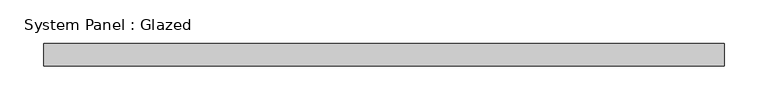
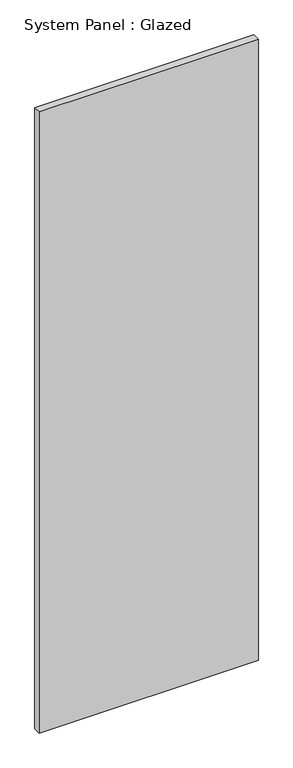
"""IFC4 building model written with IfcOpenShell, lengths in millimetres: plate geometry, System Panel : Glazed."""

from ifc_helpers import new_model, si_unit, origin, origin_with_axes, place, context, project, spatial, polyline, outline, extrude, source, transform, mapped, element, save


def system_panel_glazed_6af1fae1(model_context):
    return source(origin(), model_context, "Body", "SweptSolid", [
        extrude(outline(polyline([(387.35, 19.05), (-387.35, 19.05), (-387.35, 44.45), (387.35, 44.45), (387.35, 19.05)])), origin_with_axes(), (0.0, 0.0, 1.0), 2318.7520936),
    ])


if __name__ == "__main__":
    model = new_model("IFC4")
    model_context = context("Model", 3, world=origin())
    ifc_project = project(units=[si_unit("LENGTHUNIT", "METRE", prefix="MILLI")], contexts=[model_context])
    site = spatial("IfcSite", under=ifc_project)
    building = spatial("IfcBuilding", under=site)
    placement = place(None, origin())
    system_panel_glazed_shape = system_panel_glazed_6af1fae1(model_context)
    element("IfcPlate", 1, ObjectType="System Panel : Glazed", at=placement, inside=building, context=model_context, shape_type="MappedRepresentation", body=[
        mapped(system_panel_glazed_shape, transform((0.0, 0.0, 0.0), x_axis=(1.0, 0.0, 0.0), y_axis=(0.0, 1.0, 0.0), z_axis=(0.0, 0.0, 1.0))),
    ])
    save(model, "model.ifc")

# Revit data of these elements
# Type "System Panel : Glazed"
#   Construction Type Id = "GSP4R"
#   Analytic Construction = "1/8 in Pilkington single glazing"
#   Visual Light Transmittance = 0.9
#   Solar Heat Gain Coefficient = 0.86
#   Heat Transfer Coefficient (U) = 1.18115 BTU/(h·ft²·°F)
#   Define Thermal Properties by = 1
# Element 1 (IfcPlate, "System Panel : Glazed")
#   Materials on its faces: "Glass"
# Materials
#   "Glass": class "Glass", colour RGB 0 128 192, transparency 0.75, Description = "Soda Lime Glass", Cost = 0
